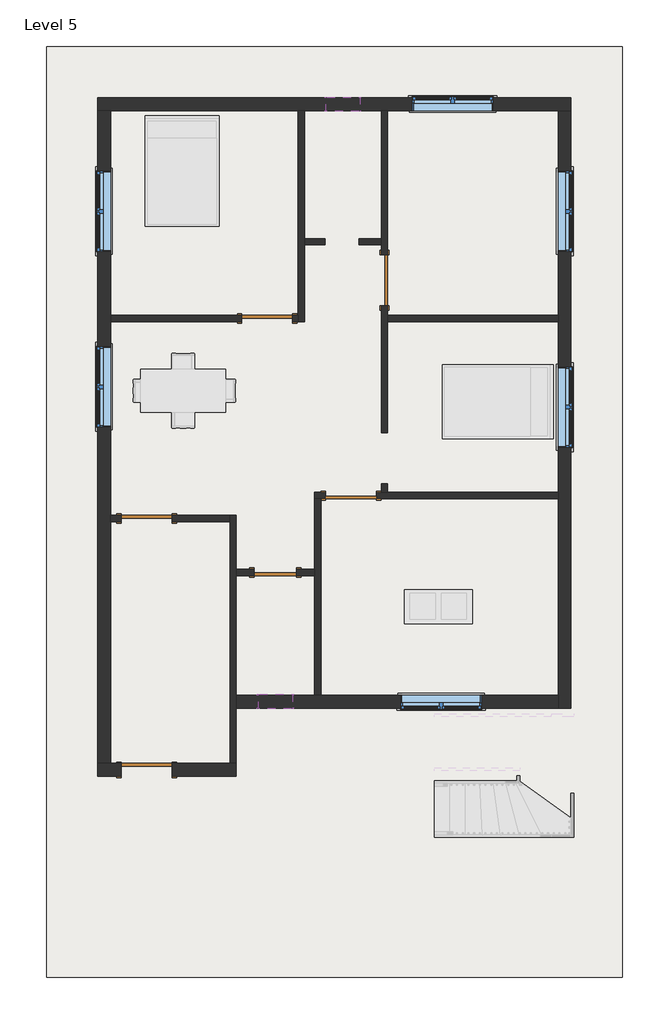
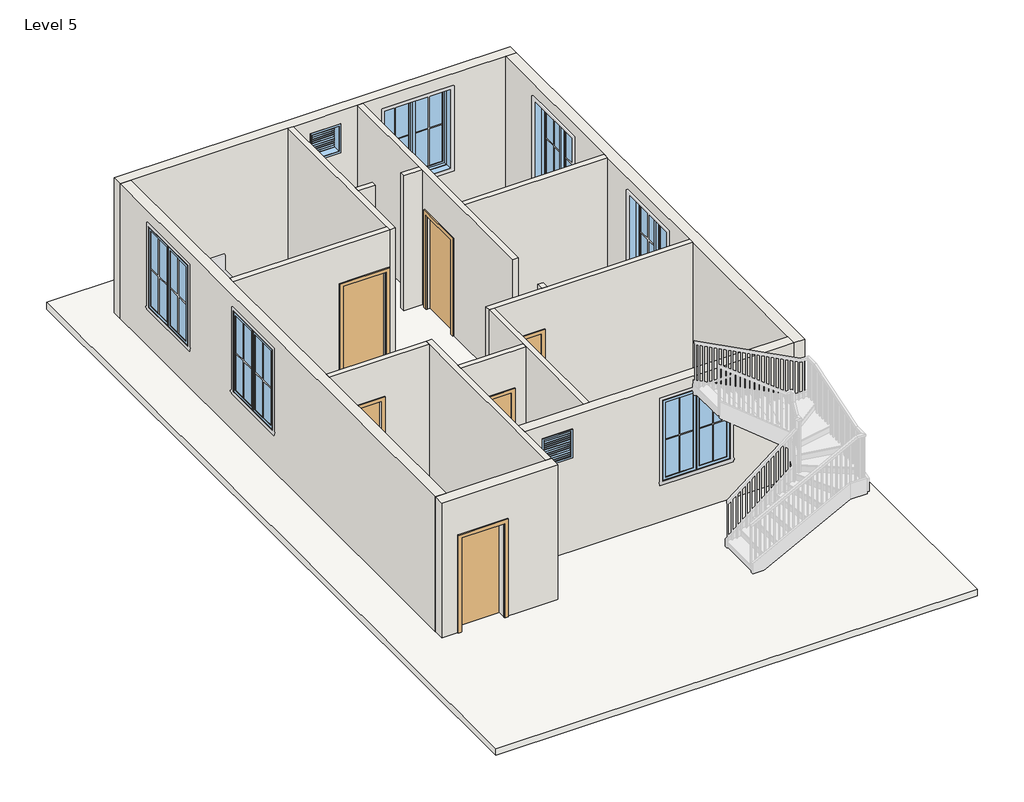
# One storey, part 1 of 3: 17 walls, 8 windows, 6 doors, 1 roof.
"""IFC4 building model written with IfcOpenShell, lengths in millimetres."""

from ifc_helpers import new_model, si_unit, frame, origin, place, context, project, spatial, polyline, outline, extrude, faceted_brep, transform, mapped, element, save
from components import door_214872d5, single_flush_door_3_e5f9f3c4, single_flush_door_3_305aa2a5, single_flush_door_3_a90ba1ad, window_9ac97e1a, window_f2d8fef0

model = new_model("IFC4")

# Units and contexts
model_context = context("Model", 3, world=origin())
ifc_project = project(units=[si_unit("LENGTHUNIT", "METRE", prefix="MILLI")], contexts=[model_context])

# Site, building, storey
site = spatial("IfcSite", under=ifc_project)
building = spatial("IfcBuilding", under=site)
storey = spatial("IfcBuildingStorey", under=building, Name="Level 5", Elevation=9601.2)

# Doors
placement = place(None, origin())
door_shape = door_214872d5(model_context)
element("IfcDoor", 1, ObjectType="Single-Flush : DOOR 2'6\"", at=placement, inside=storey, context=model_context, shape_type="MappedRepresentation", body=[
    mapped(door_shape, transform((-2309.3144966, -2885.2590409, 9601.2), x_axis=(-1.0, 0.0, 0.0), y_axis=(0.0, -1.0, 0.0), z_axis=(0.0, 0.0, 1.0))),
])
single_flush_door_3_shape = single_flush_door_3_e5f9f3c4(model_context)
element("IfcDoor", 2, ObjectType="Single-Flush : DOOR 3'", at=placement, inside=storey, context=model_context, shape_type="MappedRepresentation", body=[
    mapped(single_flush_door_3_shape, transform((-2455.3644966, 1648.6409591, 9601.2), x_axis=(1.0, 0.0, 0.0), y_axis=(0.0, 1.0, 0.0), z_axis=(0.0, 0.0, 1.0))),
])
element("IfcDoor", 3, ObjectType="Single-Flush : DOOR 3'", at=placement, inside=storey, context=model_context, shape_type="MappedRepresentation", body=[
    mapped(single_flush_door_3_shape, transform((-359.8644966, 2334.4409591, 9601.2), x_axis=(0.0, -1.0, 0.0), y_axis=(1.0, 0.0, 0.0), z_axis=(0.0, 0.0, 1.0))),
])
element("IfcDoor", 4, ObjectType="Single-Flush : DOOR 3'", at=placement, inside=storey, context=model_context, shape_type="MappedRepresentation", body=[
    mapped(single_flush_door_3_shape, transform((-956.7644966, -1513.6590409, 9601.2), x_axis=(-1.0, 0.0, 0.0), y_axis=(0.0, -1.0, 0.0), z_axis=(0.0, 0.0, 1.0))),
])
single_flush_door_3_2_shape = single_flush_door_3_305aa2a5(model_context)
element("IfcDoor", 5, ObjectType="Single-Flush : DOOR 3'", at=placement, inside=storey, context=model_context, shape_type="MappedRepresentation", body=[
    mapped(single_flush_door_3_2_shape, transform((-4608.0144966, -1920.0590409, 9601.2), x_axis=(-1.0, 0.0, 0.0), y_axis=(0.0, -1.0, 0.0), z_axis=(0.0, 0.0, 1.0))),
])
single_flush_door_3_3_shape = single_flush_door_3_a90ba1ad(model_context)
element("IfcDoor", 6, ObjectType="Single-Flush : DOOR 3'", at=placement, inside=storey, context=model_context, shape_type="MappedRepresentation", body=[
    mapped(single_flush_door_3_3_shape, transform((-4608.0144966, -6409.5090409, 9601.2), x_axis=(-1.0, 0.0, 0.0), y_axis=(0.0, -1.0, 0.0), z_axis=(0.0, 0.0, 1.0))),
])

# Roof
element("IfcRoof", 7, ObjectType="ROOF 6\"", at=placement, inside=storey, context=model_context, shape_type="SweptSolid", body=[
    extrude(outline(polyline([(-6398.7144966, 6506.3909591), (3888.2855034, 6506.3909591), (3888.2855034, -10115.6142473), (-6398.7144966, -10115.6142473), (-6398.7144966, 6506.3909591)])), frame((0.0, 0.0, 9448.8), z_axis=(0.0, 0.0, 1.0), x_axis=(1.0, 0.0, 0.0)), (0.0, 0.0, 1.0), 152.4),
])

# Walls
element("IfcWall", 8, ObjectType="WALL 4.5\"", at=placement, inside=storey, context=model_context, shape_type="Brep", body=[
    faceted_brep([(-1902.9144966, 5363.3909591, 9601.2), (-1902.9144966, 1705.7909591, 9601.2), (-1902.9144966, 1591.4909591, 9601.2), (-1902.9144966, 1591.4909591, 12649.2), (-1902.9144966, 1705.7909591, 12649.2), (-1902.9144966, 5363.3909591, 12649.2), (-1788.6144966, 5363.3909591, 9601.2), (-1788.6144966, 5363.3909591, 12649.2), (-1788.6144966, 3077.3909591, 12649.2), (-1788.6144966, 2963.0909591, 12649.2), (-1788.6144966, 1591.4909591, 12649.2), (-1788.6144966, 1591.4909591, 9601.2), (-1788.6144966, 2963.0909591, 9601.2), (-1788.6144966, 3077.3909591, 9601.2)], [[[0, 1, 2, 3, 4, 5]], [[6, 7, 8, 9, 10, 11, 12, 13]], [[2, 1, 0, 6, 13, 12, 11]], [[0, 5, 7, 6]], [[3, 2, 11, 10]], [[5, 4, 3, 10, 9, 8, 7]]]),
])
element("IfcWall", 9, ObjectType="WALL 4.5\"", at=placement, inside=storey, context=model_context, shape_type="SweptSolid", body=[
    extrude(outline(polyline([(11734.8, -1998.1644966), (9601.2, -1998.1644966), (9601.2, -1902.9144966), (12649.2, -1902.9144966), (12649.2, -5255.7144966), (9601.2, -5255.7144966), (9601.2, -2912.5644966), (11734.8, -2912.5644966), (11734.8, -1998.1644966)])), frame((0.0, 1591.4909591, 0.0), z_axis=(0.0, 1.0, 0.0), x_axis=(0.0, 0.0, 1.0)), (0.0, 0.0, 1.0), 114.3),
])
element("IfcWall", 10, ObjectType="WALL 4.5\"", at=placement, inside=storey, context=model_context, shape_type="Brep", body=[
    faceted_brep([(-417.0144966, 1877.2409591, 11734.8), (-417.0144966, 1877.2409591, 9601.2), (-417.0144966, -389.7090409, 9601.2), (-417.0144966, -389.7090409, 12649.2), (-417.0144966, 2963.0909591, 12649.2), (-417.0144966, 3077.3909591, 12649.2), (-417.0144966, 5363.3909591, 12649.2), (-417.0144966, 5363.3909591, 9601.2), (-417.0144966, 3077.3909591, 9601.2), (-417.0144966, 2963.0909591, 9601.2), (-417.0144966, 2791.6409591, 9601.2), (-417.0144966, 2791.6409591, 11734.8), (-302.7144966, -389.7090409, 9601.2), (-302.7144966, 1591.4909591, 9601.2), (-302.7144966, 1705.7909591, 9601.2), (-302.7144966, 1877.2409591, 9601.2), (-302.7144966, 1877.2409591, 11734.8), (-302.7144966, 2791.6409591, 11734.8), (-302.7144966, 2791.6409591, 9601.2), (-302.7144966, 5363.3909591, 9601.2), (-302.7144966, 5363.3909591, 12649.2), (-302.7144966, 1705.7909591, 12649.2), (-302.7144966, 1591.4909591, 12649.2), (-302.7144966, -389.7090409, 12649.2)], [[[0, 1, 2, 3, 4, 5, 6, 7, 8, 9, 10, 11]], [[12, 13, 14, 15, 16, 17, 18, 19, 20, 21, 22, 23]], [[2, 1, 15, 14, 13, 12]], [[10, 9, 8, 7, 19, 18]], [[3, 2, 12, 23]], [[7, 6, 20, 19]], [[16, 15, 1, 0]], [[17, 16, 0, 11]], [[18, 17, 11, 10]], [[6, 5, 4, 3, 23, 22, 21, 20]]]),
])
element("IfcWall", 11, ObjectType="WALL 4.5\"", at=placement, inside=storey, context=model_context, shape_type="SweptSolid", body=[
    extrude(outline(polyline([(-302.7144966, 1705.7909591), (2745.2855034, 1705.7909591), (2745.2855034, 1591.4909591), (-302.7144966, 1591.4909591), (-302.7144966, 1705.7909591)])), frame((0.0, 0.0, 9601.2), z_axis=(0.0, 0.0, 1.0), x_axis=(1.0, 0.0, 0.0)), (0.0, 0.0, 1.0), 3048.0),
])
element("IfcWall", 12, ObjectType="WALL 4.5\"", at=placement, inside=storey, context=model_context, shape_type="SweptSolid", body=[
    extrude(outline(polyline([(-1423.1234474, 2963.0909591), (-1788.6144966, 2963.0909591), (-1788.6144966, 3077.3909591), (-1423.1234474, 3077.3909591), (-1423.1234474, 2963.0909591)])), frame((0.0, 0.0, 9601.2), z_axis=(0.0, 0.0, 1.0), x_axis=(1.0, 0.0, 0.0)), (0.0, 0.0, 1.0), 3048.0),
])
element("IfcWall", 13, ObjectType="WALL 4.5\"", at=placement, inside=storey, context=model_context, shape_type="Brep", body=[
    faceted_brep([(-1413.9644966, -1456.5090409, 11734.8), (-1413.9644966, -1456.5090409, 9601.2), (-1610.8144966, -1456.5090409, 9601.2), (-1610.8144966, -1456.5090409, 12649.2), (-417.0144966, -1456.5090409, 12649.2), (-302.7144966, -1456.5090409, 12649.2), (2745.2855034, -1456.5090409, 12649.2), (2745.2855034, -1456.5090409, 9601.2), (-302.7144966, -1456.5090409, 9601.2), (-417.0144966, -1456.5090409, 9601.2), (-499.5644966, -1456.5090409, 9601.2), (-499.5644966, -1456.5090409, 11734.8), (-1610.8144966, -1570.8090409, 9601.2), (-1496.5144966, -1570.8090409, 9601.2), (-1413.9644966, -1570.8090409, 9601.2), (-1413.9644966, -1570.8090409, 11734.8), (-499.5644966, -1570.8090409, 11734.8), (-499.5644966, -1570.8090409, 9601.2), (2745.2855034, -1570.8090409, 9601.2), (2745.2855034, -1570.8090409, 12649.2), (-1496.5144966, -1570.8090409, 12649.2), (-1610.8144966, -1570.8090409, 12649.2)], [[[0, 1, 2, 3, 4, 5, 6, 7, 8, 9, 10, 11]], [[12, 13, 14, 15, 16, 17, 18, 19, 20, 21]], [[2, 1, 14, 13, 12]], [[10, 9, 8, 7, 18, 17]], [[7, 6, 19, 18]], [[3, 2, 12, 21]], [[15, 14, 1, 0]], [[16, 15, 0, 11]], [[17, 16, 11, 10]], [[6, 5, 4, 3, 21, 20, 19]]]),
])
element("IfcWall", 14, ObjectType="WALL 4.5\"", at=placement, inside=storey, context=model_context, shape_type="SweptSolid", body=[
    extrude(outline(polyline([(-302.7144966, -1304.1090409), (-302.7144966, -1456.5090409), (-417.0144966, -1456.5090409), (-417.0144966, -1304.1090409), (-302.7144966, -1304.1090409)])), frame((0.0, 0.0, 9601.2), z_axis=(0.0, 0.0, 1.0), x_axis=(1.0, 0.0, 0.0)), (0.0, 0.0, 1.0), 3048.0),
])
element("IfcWall", 15, ObjectType="WALL 4.5\"", at=placement, inside=storey, context=model_context, shape_type="Brep", body=[
    faceted_brep([(-1610.8144966, -1570.8090409, 9601.2), (-1610.8144966, -2828.1090409, 9601.2), (-1610.8144966, -2942.4090409, 9601.2), (-1610.8144966, -5076.0090409, 9601.2), (-1610.8144966, -5076.0090409, 12649.2), (-1610.8144966, -2942.4090409, 12649.2), (-1610.8144966, -2828.1090409, 12649.2), (-1610.8144966, -1570.8090409, 12649.2), (-1496.5144966, -1570.8090409, 9601.2), (-1496.5144966, -1570.8090409, 12649.2), (-1496.5144966, -5076.0090409, 12649.2), (-1496.5144966, -5076.0090409, 9601.2)], [[[0, 1, 2, 3, 4, 5, 6, 7]], [[8, 9, 10, 11]], [[3, 2, 1, 0, 8, 11]], [[0, 7, 9, 8]], [[4, 3, 11, 10]], [[7, 6, 5, 4, 10, 9]]]),
])
element("IfcWall", 16, ObjectType="WALL 4.5\"", at=placement, inside=storey, context=model_context, shape_type="SweptSolid", body=[
    extrude(outline(polyline([(9601.2, -3007.8144966), (9601.2, -2690.3144966), (11734.8, -2690.3144966), (11734.8, -1928.3144966), (9601.2, -1928.3144966), (9601.2, -1610.8144966), (12649.2, -1610.8144966), (12649.2, -3007.8144966), (9601.2, -3007.8144966)])), frame((0.0, -2942.4090409, 0.0), z_axis=(0.0, 1.0, 0.0), x_axis=(0.0, 0.0, 1.0)), (0.0, 0.0, 1.0), 114.3),
])
element("IfcWall", 17, ObjectType="WALL 4.5\"", at=placement, inside=storey, context=model_context, shape_type="Brep", body=[
    faceted_brep([(-3007.8144966, -6295.2090409, 9601.2), (-3007.8144966, -5304.6090409, 9601.2), (-3007.8144966, -5076.0090409, 9601.2), (-3007.8144966, -2942.4090409, 9601.2), (-3007.8144966, -2828.1090409, 9601.2), (-3007.8144966, -1862.9090409, 9601.2), (-3007.8144966, -1862.9090409, 12649.2), (-3007.8144966, -2828.1090409, 12649.2), (-3007.8144966, -2942.4090409, 12649.2), (-3007.8144966, -5076.0090409, 12649.2), (-3007.8144966, -5304.6090409, 12649.2), (-3007.8144966, -6295.2090409, 12649.2), (-3122.1144966, -6295.2090409, 9601.2), (-3122.1144966, -6295.2090409, 12649.2), (-3122.1144966, -1977.2090409, 12649.2), (-3122.1144966, -1862.9090409, 12649.2), (-3122.1144966, -1862.9090409, 9601.2), (-3122.1144966, -1977.2090409, 9601.2)], [[[0, 1, 2, 3, 4, 5, 6, 7, 8, 9, 10, 11]], [[12, 13, 14, 15, 16, 17]], [[5, 4, 3, 2, 1, 0, 12, 17, 16]], [[0, 11, 13, 12]], [[6, 5, 16, 15]], [[11, 10, 9, 8, 7, 6, 15, 14, 13]]]),
])
element("IfcWall", 18, ObjectType="WALL 4.5\"", at=placement, inside=storey, context=model_context, shape_type="SweptSolid", body=[
    extrude(outline(polyline([(9601.2, -5255.7144966), (9601.2, -5065.2144966), (11734.8, -5065.2144966), (11734.8, -4150.8144966), (9601.2, -4150.8144966), (9601.2, -3122.1144966), (12649.2, -3122.1144966), (12649.2, -5255.7144966), (9601.2, -5255.7144966)])), frame((0.0, -1977.2090409, 0.0), z_axis=(0.0, 1.0, 0.0), x_axis=(0.0, 0.0, 1.0)), (0.0, 0.0, 1.0), 114.3),
])
element("IfcWall", 19, ObjectType="WALL 4.5\"", at=placement, inside=storey, context=model_context, shape_type="SweptSolid", body=[
    extrude(outline(polyline([(-417.0144966, 2963.0909591), (-814.3659123, 2963.0909591), (-814.3659123, 3077.3909591), (-417.0144966, 3077.3909591), (-417.0144966, 2963.0909591)])), frame((0.0, 0.0, 9601.2), z_axis=(0.0, 0.0, 1.0), x_axis=(1.0, 0.0, 0.0)), (0.0, 0.0, 1.0), 3048.0),
])
element("IfcWall", 20, ObjectType="WALL 9\"", at=placement, inside=storey, context=model_context, shape_type="Brep", body=[
    faceted_brep([(-5484.3144966, 5363.3909591, 9601.2), (-5255.7144966, 5363.3909591, 9601.2), (-1902.9144966, 5363.3909591, 9601.2), (-1788.6144966, 5363.3909591, 9601.2), (-417.0144966, 5363.3909591, 9601.2), (-302.7144966, 5363.3909591, 9601.2), (2745.2855034, 5363.3909591, 9601.2), (2973.8855034, 5363.3909591, 9601.2), (2973.8855034, 5363.3909591, 12649.2), (2745.2855034, 5363.3909591, 12649.2), (-302.7144966, 5363.3909591, 12649.2), (-417.0144966, 5363.3909591, 12649.2), (-1788.6144966, 5363.3909591, 12649.2), (-1902.9144966, 5363.3909591, 12649.2), (-5255.7144966, 5363.3909591, 12649.2), (-5484.3144966, 5363.3909591, 12649.2), (1583.2355034, 5363.3909591, 12344.4), (1583.2355034, 5363.3909591, 10515.6), (135.4355034, 5363.3909591, 10515.6), (135.4355034, 5363.3909591, 12344.4), (-1407.6144966, 5363.3909591, 12344.4), (-798.0144966, 5363.3909591, 12344.4), (-798.0144966, 5363.3909591, 11734.8), (-1407.6144966, 5363.3909591, 11734.8), (-5484.3144966, 5591.9909591, 9601.2), (-5484.3144966, 5591.9909591, 12649.2), (2973.8855034, 5591.9909591, 12649.2), (2973.8855034, 5591.9909591, 9601.2), (1583.2355034, 5591.9909591, 12344.4), (135.4355034, 5591.9909591, 12344.4), (135.4355034, 5591.9909591, 10515.6), (1583.2355034, 5591.9909591, 10515.6), (-1407.6144966, 5591.9909591, 12344.4), (-1407.6144966, 5591.9909591, 11734.8), (-798.0144966, 5591.9909591, 11734.8), (-798.0144966, 5591.9909591, 12344.4)], [[[0, 1, 2, 3, 4, 5, 6, 7, 8, 9, 10, 11, 12, 13, 14, 15], [16, 17, 18, 19], [20, 21, 22, 23]], [[24, 25, 26, 27], [28, 29, 30, 31], [32, 33, 34, 35]], [[7, 6, 5, 4, 3, 2, 1, 0, 24, 27]], [[8, 7, 27, 26]], [[0, 15, 25, 24]], [[17, 16, 28, 31]], [[18, 17, 31, 30]], [[19, 18, 30, 29]], [[16, 19, 29, 28]], [[33, 32, 20, 23]], [[34, 33, 23, 22]], [[35, 34, 22, 21]], [[32, 35, 21, 20]], [[15, 14, 13, 12, 11, 10, 9, 8, 26, 25]]]),
])
element("IfcWall", 21, ObjectType="WALL 9\"", at=placement, inside=storey, context=model_context, shape_type="Brep", body=[
    faceted_brep([(2745.2855034, 5363.3909591, 9601.2), (2745.2855034, 1705.7909591, 9601.2), (2745.2855034, 1591.4909591, 9601.2), (2745.2855034, -1456.5090409, 9601.2), (2745.2855034, -1570.8090409, 9601.2), (2745.2855034, -5076.0090409, 9601.2), (2745.2855034, -5304.6090409, 9601.2), (2745.2855034, -5304.6090409, 12649.2), (2745.2855034, -5076.0090409, 12649.2), (2745.2855034, -1570.8090409, 12649.2), (2745.2855034, -1456.5090409, 12649.2), (2745.2855034, 1591.4909591, 12649.2), (2745.2855034, 1705.7909591, 12649.2), (2745.2855034, 5363.3909591, 12649.2), (2745.2855034, -656.4090409, 12344.4), (2745.2855034, -656.4090409, 10515.6), (2745.2855034, 791.3909591, 10515.6), (2745.2855034, 791.3909591, 12344.4), (2745.2855034, 2839.2659591, 12344.4), (2745.2855034, 2839.2659591, 10515.6), (2745.2855034, 4287.0659591, 10515.6), (2745.2855034, 4287.0659591, 12344.4), (2973.8855034, 5363.3909591, 9601.2), (2973.8855034, 5363.3909591, 12649.2), (2973.8855034, -5304.6090409, 12649.2), (2973.8855034, -5304.6090409, 9601.2), (2973.8855034, -656.4090409, 12344.4), (2973.8855034, 791.3909591, 12344.4), (2973.8855034, 791.3909591, 10515.6), (2973.8855034, -656.4090409, 10515.6), (2973.8855034, 2839.2659591, 12344.4), (2973.8855034, 4287.0659591, 12344.4), (2973.8855034, 4287.0659591, 10515.6), (2973.8855034, 2839.2659591, 10515.6)], [[[0, 1, 2, 3, 4, 5, 6, 7, 8, 9, 10, 11, 12, 13], [14, 15, 16, 17], [18, 19, 20, 21]], [[22, 23, 24, 25], [26, 27, 28, 29], [30, 31, 32, 33]], [[6, 5, 4, 3, 2, 1, 0, 22, 25]], [[0, 13, 23, 22]], [[7, 6, 25, 24]], [[15, 14, 26, 29]], [[16, 15, 29, 28]], [[17, 16, 28, 27]], [[14, 17, 27, 26]], [[19, 18, 30, 33]], [[20, 19, 33, 32]], [[21, 20, 32, 31]], [[18, 21, 31, 30]], [[13, 12, 11, 10, 9, 8, 7, 24, 23]]]),
])
element("IfcWall", 22, ObjectType="WALL 9\"", at=placement, inside=storey, context=model_context, shape_type="Brep", body=[
    faceted_brep([(2745.2855034, -5076.0090409, 9601.2), (-1496.5144966, -5076.0090409, 9601.2), (-1610.8144966, -5076.0090409, 9601.2), (-3007.8144966, -5076.0090409, 9601.2), (-3007.8144966, -5076.0090409, 12649.2), (-1610.8144966, -5076.0090409, 12649.2), (-1496.5144966, -5076.0090409, 12649.2), (2745.2855034, -5076.0090409, 12649.2), (-70.9394966, -5076.0090409, 12344.4), (-70.9394966, -5076.0090409, 10515.6), (1376.8605034, -5076.0090409, 10515.6), (1376.8605034, -5076.0090409, 12344.4), (-2004.5144966, -5076.0090409, 12344.4), (-2614.1144966, -5076.0090409, 12344.4), (-2614.1144966, -5076.0090409, 11734.8), (-2004.5144966, -5076.0090409, 11734.8), (2745.2855034, -5304.6090409, 9601.2), (2745.2855034, -5304.6090409, 12649.2), (-3007.8144966, -5304.6090409, 12649.2), (-3007.8144966, -5304.6090409, 9601.2), (-70.9394966, -5304.6090409, 12344.4), (1376.8605034, -5304.6090409, 12344.4), (1376.8605034, -5304.6090409, 10515.6), (-70.9394966, -5304.6090409, 10515.6), (-2004.5144966, -5304.6090409, 12344.4), (-2004.5144966, -5304.6090409, 11734.8), (-2614.1144966, -5304.6090409, 11734.8), (-2614.1144966, -5304.6090409, 12344.4)], [[[0, 1, 2, 3, 4, 5, 6, 7], [8, 9, 10, 11], [12, 13, 14, 15]], [[16, 17, 18, 19], [20, 21, 22, 23], [24, 25, 26, 27]], [[3, 2, 1, 0, 16, 19]], [[0, 7, 17, 16]], [[4, 3, 19, 18]], [[9, 8, 20, 23]], [[10, 9, 23, 22]], [[11, 10, 22, 21]], [[8, 11, 21, 20]], [[25, 24, 12, 15]], [[26, 25, 15, 14]], [[27, 26, 14, 13]], [[24, 27, 13, 12]], [[7, 6, 5, 4, 18, 17]]]),
])
element("IfcWall", 23, ObjectType="WALL 9\"", at=placement, inside=storey, context=model_context, shape_type="Brep", body=[
    faceted_brep([(-5065.2144966, -6295.2090409, 11734.8), (-5065.2144966, -6295.2090409, 9601.2), (-5255.7144966, -6295.2090409, 9601.2), (-5484.3144966, -6295.2090409, 9601.2), (-5484.3144966, -6295.2090409, 12649.2), (-5255.7144966, -6295.2090409, 12649.2), (-3122.1144966, -6295.2090409, 12649.2), (-3007.8144966, -6295.2090409, 12649.2), (-3007.8144966, -6295.2090409, 9601.2), (-3122.1144966, -6295.2090409, 9601.2), (-4150.8144966, -6295.2090409, 9601.2), (-4150.8144966, -6295.2090409, 11734.8), (-5484.3144966, -6523.8090409, 9601.2), (-5065.2144966, -6523.8090409, 9601.2), (-5065.2144966, -6523.8090409, 11734.8), (-4150.8144966, -6523.8090409, 11734.8), (-4150.8144966, -6523.8090409, 9601.2), (-3007.8144966, -6523.8090409, 9601.2), (-3007.8144966, -6523.8090409, 12649.2), (-5484.3144966, -6523.8090409, 12649.2)], [[[0, 1, 2, 3, 4, 5, 6, 7, 8, 9, 10, 11]], [[12, 13, 14, 15, 16, 17, 18, 19]], [[10, 9, 8, 17, 16]], [[3, 2, 1, 13, 12]], [[4, 3, 12, 19]], [[8, 7, 18, 17]], [[7, 6, 5, 4, 19, 18]], [[14, 13, 1, 0]], [[15, 14, 0, 11]], [[16, 15, 11, 10]]]),
])
element("IfcWall", 24, ObjectType="WALL 9\"", at=placement, inside=storey, context=model_context, shape_type="Brep", body=[
    faceted_brep([(-5255.7144966, -6295.2090409, 9601.2), (-5255.7144966, -1977.2090409, 9601.2), (-5255.7144966, -1862.9090409, 9601.2), (-5255.7144966, 1591.4909591, 9601.2), (-5255.7144966, 1705.7909591, 9601.2), (-5255.7144966, 5363.3909591, 9601.2), (-5255.7144966, 5363.3909591, 12649.2), (-5255.7144966, 1705.7909591, 12649.2), (-5255.7144966, 1591.4909591, 12649.2), (-5255.7144966, -1862.9090409, 12649.2), (-5255.7144966, -1977.2090409, 12649.2), (-5255.7144966, -6295.2090409, 12649.2), (-5255.7144966, 4287.0659591, 12344.4), (-5255.7144966, 4287.0659591, 10515.6), (-5255.7144966, 2839.2659591, 10515.6), (-5255.7144966, 2839.2659591, 12344.4), (-5255.7144966, 1153.3409591, 12344.4), (-5255.7144966, 1153.3409591, 10515.6), (-5255.7144966, -294.4590409, 10515.6), (-5255.7144966, -294.4590409, 12344.4), (-5484.3144966, -6295.2090409, 9601.2), (-5484.3144966, -6295.2090409, 12649.2), (-5484.3144966, 5363.3909591, 12649.2), (-5484.3144966, 5363.3909591, 9601.2), (-5484.3144966, 4287.0659591, 12344.4), (-5484.3144966, 2839.2659591, 12344.4), (-5484.3144966, 2839.2659591, 10515.6), (-5484.3144966, 4287.0659591, 10515.6), (-5484.3144966, 1153.3409591, 12344.4), (-5484.3144966, -294.4590409, 12344.4), (-5484.3144966, -294.4590409, 10515.6), (-5484.3144966, 1153.3409591, 10515.6)], [[[0, 1, 2, 3, 4, 5, 6, 7, 8, 9, 10, 11], [12, 13, 14, 15], [16, 17, 18, 19]], [[20, 21, 22, 23], [24, 25, 26, 27], [28, 29, 30, 31]], [[5, 4, 3, 2, 1, 0, 20, 23]], [[0, 11, 21, 20]], [[6, 5, 23, 22]], [[13, 12, 24, 27]], [[14, 13, 27, 26]], [[15, 14, 26, 25]], [[12, 15, 25, 24]], [[17, 16, 28, 31]], [[18, 17, 31, 30]], [[19, 18, 30, 29]], [[16, 19, 29, 28]], [[11, 10, 9, 8, 7, 6, 22, 21]]]),
])

# Windows
window_shape = window_9ac97e1a(model_context)
element("IfcWindow", 25, ObjectType="Window-Casement-Double : 57\" x 72\"", at=placement, inside=storey, context=model_context, shape_type="MappedRepresentation", body=[
    mapped(window_shape, transform((2859.5855034, 67.4909591, 9601.2), x_axis=(0.0, -1.0, 0.0), y_axis=(1.0, 0.0, 0.0), z_axis=(0.0, 0.0, 1.0))),
])
element("IfcWindow", 26, ObjectType="Window-Casement-Double : 57\" x 72\"", at=placement, inside=storey, context=model_context, shape_type="MappedRepresentation", body=[
    mapped(window_shape, transform((2859.5855034, 3563.1659591, 9601.2), x_axis=(0.0, -1.0, 0.0), y_axis=(1.0, 0.0, 0.0), z_axis=(0.0, 0.0, 1.0))),
])
element("IfcWindow", 27, ObjectType="Window-Casement-Double : 57\" x 72\"", at=placement, inside=storey, context=model_context, shape_type="MappedRepresentation", body=[
    mapped(window_shape, transform((859.3355034, 5477.6909591, 9601.2), x_axis=(1.0, 0.0, 0.0), y_axis=(0.0, 1.0, 0.0), z_axis=(0.0, 0.0, 1.0))),
])
element("IfcWindow", 28, ObjectType="Window-Casement-Double : 57\" x 72\"", at=placement, inside=storey, context=model_context, shape_type="MappedRepresentation", body=[
    mapped(window_shape, transform((-5370.0144966, 3563.1659591, 9601.2), x_axis=(0.0, 1.0, 0.0), y_axis=(-1.0, 0.0, 0.0), z_axis=(0.0, 0.0, 1.0))),
])
element("IfcWindow", 29, ObjectType="Window-Casement-Double : 57\" x 72\"", at=placement, inside=storey, context=model_context, shape_type="MappedRepresentation", body=[
    mapped(window_shape, transform((-5370.0144966, 429.4409591, 9601.2), x_axis=(0.0, 1.0, 0.0), y_axis=(-1.0, 0.0, 0.0), z_axis=(0.0, 0.0, 1.0))),
])
element("IfcWindow", 30, ObjectType="Window-Casement-Double : 57\" x 72\"", at=placement, inside=storey, context=model_context, shape_type="MappedRepresentation", body=[
    mapped(window_shape, transform((652.9605034, -5190.3090409, 9601.2), x_axis=(-1.0, 0.0, 0.0), y_axis=(0.0, -1.0, 0.0), z_axis=(0.0, 0.0, 1.0))),
])
window_2_shape = window_f2d8fef0(model_context)
element("IfcWindow", 31, ObjectType="Window-Louvers : 24\" x 24\"", at=placement, inside=storey, context=model_context, shape_type="MappedRepresentation", body=[
    mapped(window_2_shape, transform((-1102.8144966, 5484.0409591, 10820.4), x_axis=(1.0, 0.0, 0.0), y_axis=(0.0, 1.0, 0.0), z_axis=(0.0, 0.0, 1.0))),
])
element("IfcWindow", 32, ObjectType="Window-Louvers : 24\" x 24\"", at=placement, inside=storey, context=model_context, shape_type="MappedRepresentation", body=[
    mapped(window_2_shape, transform((-2309.3144966, -5196.6590409, 10820.4), x_axis=(-1.0, 0.0, 0.0), y_axis=(0.0, -1.0, 0.0), z_axis=(0.0, 0.0, 1.0))),
])

save(model, "model.ifc")

# Revit data of these elements
# Type "Single-Flush : DOOR 2'6\""
#   Type Mark = "10"
#   Construction Type Id = "MDOOR"
#   Assembly Code = "C1020"
#   Analytic Construction = "Metal"
#   Thickness = 0' - 2"
#   Heat Transfer Coefficient (U) = 0.651978 BTU/(h·ft²·°F)
#   Height = 7' - 0"
#   Trim Projection Ext = 0' - 1"
#   Trim Projection Int = 0' - 1"
#   Trim Width = 0' - 3"
#   Width = 2' - 6"
#   Define Thermal Properties by = 1
#   Door Material = Door - Panel
#   Frame Material = Door - Frame
#   Visual Light Transmittance = 0
#   Solar Heat Gain Coefficient = 0
#   Function = (empty or 0)
#   Wall Closure = (empty or 0)
# Type "Single-Flush : DOOR 3'"
#   Type Mark = "9"
#   Construction Type Id = "MDOOR"
#   Assembly Code = "C1020"
#   Analytic Construction = "Metal"
#   Thickness = 0' - 2"
#   Heat Transfer Coefficient (U) = 0.651978 BTU/(h·ft²·°F)
#   Height = 7' - 0"
#   Trim Projection Ext = 0' - 1"
#   Trim Projection Int = 0' - 1"
#   Trim Width = 0' - 3"
#   Width = 3' - 0"
#   Define Thermal Properties by = 1
#   Door Material = Door - Panel
#   Frame Material = Door - Frame
#   Visual Light Transmittance = 0
#   Solar Heat Gain Coefficient = 0
#   Function = (empty or 0)
#   Wall Closure = (empty or 0)
# Type "ROOF 6\""
#   Assembly Code = "B1020"
#   Layers, outside or top first: 0' - 6" no material (function 1)
# Type "WALL 4.5\""
#   Assembly Code = "B2010"
#   Layers, outside or top first: 0' - 4 1/2" no material (function 1)
# Type "WALL 9\""
#   Assembly Code = "B2010"
#   Layers, outside or top first: 0' - 9" no material (function 1)
# Type "Window-Casement-Double : 57\" x 72\""
#   Type Mark = "17"
#   Fire Rating = "0.5h"
#   Assembly Code = "B2020100"
#   Analytic Construction = "Double glazing - domestic"
#   Frame Extension [instance default] = 0' - 0 1/4"
#   Window Inset [instance default] = 0' - 0"
#   Wall Thickness [instance default] = 0' - 6"
#   Interior Wall Closure [instance default] = 0' - 2 1/4"
#   Half Width = 2' - 4 1/2"
#   Visual Light Transmittance = 0.81
#   Thermal Resistance (R) = 1.8146 (h·ft²·°F)/BTU
#   Solar Heat Gain Coefficient = 0.76
#   Rough Width = 4' - 9 1/2"
#   Rough Height = 6' - 0 1/2"
#   Height = 6' - 0"
#   Heat Transfer Coefficient (U) = 0.5511 BTU/(h·ft²·°F)
#   Exterior Wall Closure [instance default] = 0' - 1 1/4"
#   Extension Jamb [instance default] = 0' - 2 1/4"
#   Default Sill Height = 3' - 0"
#   Width = 4' - 9"
#   Define Thermal Properties by = 0
#   Muntin Visibility = yes
#   Interior Trim Visibility [instance default] = yes
#   Exterior Trim Visibility [instance default] = yes
#   Extension Jamb Visibility [instance default] = yes
#   Interior Trim Material = Wood - Stained
#   Muntin Pattern = Muntin Pattern_2x2 : Muntin Pattern_2x2
#   Interior Trim = Trim-Window-Interior-Flat : Picture Frame
#   Interior Frame Material = Wood - Stained
#   Glass Panel Material = Glass
#   Exterior Trim Material = Clad - White
#   Exterior Trim = Trim-Window-Exterior-Flat : with Sill
#   Exterior Frame Material = Clad - White
#   Wall Closure = (empty or 0)
# Type "Window-Louvers : 24\" x 24\""
#   Type Mark = "18"
#   Construction Type Id = "GSP4R"
#   Assembly Code = "B20"
#   Analytic Construction = "1/8 in Pilkington single glazing"
#   Visual Light Transmittance = 0.9
#   Thermal Resistance (R) = 1.53941 (h·ft²·°F)/BTU
#   Solar Heat Gain Coefficient = 0.78
#   Max Height = 1' - 11.74264"
#   Height = 2' - 0"
#   Heat Transfer Coefficient (U) = 0.6496 BTU/(h·ft²·°F)
#   Blade Width [instance default] = 1' - 10 1/2"
#   Blade Vertical Thickness = 0' - 0.35355"
#   Blade Thickness = 0' - 0 1/4"
#   Blade Spacing = 0' - 1 1/2"
#   Blade Height = 0' - 1.85355"
#   Blade Depth = 0' - 3"
#   Blade Angle = 45.00°
#   Default Sill Height = 3' - 0"
#   Trim Projection_Exterior = 0' - 0 1/2"
#   Trim Projection_Interior = 0' - 0 1/2"
#   Trim Width_Exterior = 0' - 1 1/2"
#   Trim Width_Interior = 0' - 1 1/2"
#   Width = 2' - 0"
#   Max Blade Count = 12
#   Define Thermal Properties by = 1
#   Blade Count = 12
#   Frame Material = Birch
#   Louver Material = Birch
#   Trim Exterior Material = Birch
#   Trim Interior Material = Birch
#   Wall Closure = (empty or 0)
# Element 1 (IfcDoor, "Single-Flush : DOOR 2'6\"")
#   Phase Created = New Construction
#   Materials on its faces: "Door - Frame", "Door - Panel"
# Elements 2, 3, 4, 5, 6 (IfcDoor, "Single-Flush : DOOR 3'")
#   Phase Created = New Construction
#   Materials on its faces: "Door - Frame", "Door - Panel"
# Element 7 (IfcRoof, "ROOF 6\"")
#   built-in parameter 1001705 = 31.5 (stored number, unit not read)
#   built-in parameter 1001701 = -0.5 (stored number, unit not read)
#   built-in parameter 1001710 = 33615
#   Phase Created = New Construction
#   Materials on its faces: "Cherry", "Default Roof", "Softwood, Lumber"
# Elements 8, 9, 10, 11, 12, 13, 14, 15, 16, 17, 18, 19 (IfcWall, "WALL 4.5\"")
#   Top Offset = 0' - 0"
#   Base Offset = 0' - 0"
#   Unconnected Height = 10' - 0"
#   wall height = 10' - 0"
#   Phase Created = New Construction
#   Base Constraint = Level 5
#   Materials on its faces: "Default Wall"
# Elements 20, 21, 22, 23, 24 (IfcWall, "WALL 9\"")
#   Top Offset = 0' - 0"
#   Base Offset = 0' - 0"
#   Unconnected Height = 10' - 0"
#   wall height = 10' - 0"
#   Phase Created = New Construction
#   Base Constraint = Level 5
#   Materials on its faces: "Default Wall"
# Element 25 (IfcWindow, "Window-Casement-Double : 57\" x 72\"")
#   Mark = "25"
#   Window Inset = 0' - 0"
#   Interior Wall Closure = 0' - 2 1/4"
#   Frame Extension = 0' - 0 1/4"
#   Exterior Wall Closure = 0' - 1 1/4"
#   Interior Trim Visibility = yes
#   Exterior Trim Visibility = yes
#   Phase Created = New Construction
#   Materials on its faces: "Wood - Stained", "Glass", "Clad - White"
# Element 26 (IfcWindow, "Window-Casement-Double : 57\" x 72\"")
#   Mark = "26"
#   Window Inset = 0' - 0"
#   Interior Wall Closure = 0' - 2 1/4"
#   Frame Extension = 0' - 0 1/4"
#   Exterior Wall Closure = 0' - 1 1/4"
#   Interior Trim Visibility = yes
#   Exterior Trim Visibility = yes
#   Phase Created = New Construction
#   Materials on its faces: "Wood - Stained", "Glass", "Clad - White"
# Element 27 (IfcWindow, "Window-Casement-Double : 57\" x 72\"")
#   Mark = "27"
#   Window Inset = 0' - 0"
#   Interior Wall Closure = 0' - 2 1/4"
#   Frame Extension = 0' - 0 1/4"
#   Exterior Wall Closure = 0' - 1 1/4"
#   Interior Trim Visibility = yes
#   Exterior Trim Visibility = yes
#   Phase Created = New Construction
#   Materials on its faces: "Wood - Stained", "Glass", "Clad - White"
# Element 28 (IfcWindow, "Window-Casement-Double : 57\" x 72\"")
#   Mark = "28"
#   Window Inset = 0' - 0"
#   Interior Wall Closure = 0' - 2 1/4"
#   Frame Extension = 0' - 0 1/4"
#   Exterior Wall Closure = 0' - 1 1/4"
#   Interior Trim Visibility = yes
#   Exterior Trim Visibility = yes
#   Phase Created = New Construction
#   Materials on its faces: "Wood - Stained", "Glass", "Clad - White"
# Element 29 (IfcWindow, "Window-Casement-Double : 57\" x 72\"")
#   Mark = "29"
#   Window Inset = 0' - 0"
#   Interior Wall Closure = 0' - 2 1/4"
#   Frame Extension = 0' - 0 1/4"
#   Exterior Wall Closure = 0' - 1 1/4"
#   Interior Trim Visibility = yes
#   Exterior Trim Visibility = yes
#   Phase Created = New Construction
#   Materials on its faces: "Wood - Stained", "Glass", "Clad - White"
# Element 30 (IfcWindow, "Window-Casement-Double : 57\" x 72\"")
#   Mark = "30"
#   Window Inset = 0' - 0"
#   Interior Wall Closure = 0' - 2 1/4"
#   Frame Extension = 0' - 0 1/4"
#   Exterior Wall Closure = 0' - 1 1/4"
#   Interior Trim Visibility = yes
#   Exterior Trim Visibility = yes
#   Phase Created = New Construction
#   Materials on its faces: "Wood - Stained", "Glass", "Clad - White"
# Element 31 (IfcWindow, "Window-Louvers : 24\" x 24\"")
#   Mark = "31"
#   Blade Width = 1' - 10 1/2"
#   Phase Created = New Construction
#   Materials on its faces: "Birch"
# Element 32 (IfcWindow, "Window-Louvers : 24\" x 24\"")
#   Mark = "32"
#   Blade Width = 1' - 10 1/2"
#   Phase Created = New Construction
#   Materials on its faces: "Birch"
# Materials
#   "Door - Panel": class "Wood", colour RGB 210 159 95, transparency 0, Cost = 0
#   "Door - Frame": colour RGB 118 70 51, transparency 0, Cost = 0
#   "Wood - Stained": class "Wood", colour RGB 224 178 126, transparency 0, Cost = 0
#   "Glass": class "Glass", colour RGB 0 128 192, transparency 0.75, Description = "Soda Lime Glass", Cost = 0
#   "Clad - White": class "Wood", colour RGB 242 242 238, transparency 0, Cost = 0
#   "Birch": class "Wood", colour RGB 224 178 126, transparency 0, Description = "Betula Alleghaniensis", Cost = 0
#   "Cherry": class "Wood", colour RGB 226 177 128, transparency 0, Description = "Prunus Serotina", Cost = 0
#   "Default Roof": colour RGB 88 101 114, transparency 0, Cost = 0
#   "Softwood, Lumber": class "Wood", colour RGB 223 192 134, transparency 0, Description = "Pinus Echinata", Cost = 0
#   "Default Wall": colour RGB 128 128 128, transparency 0, Cost = 0
